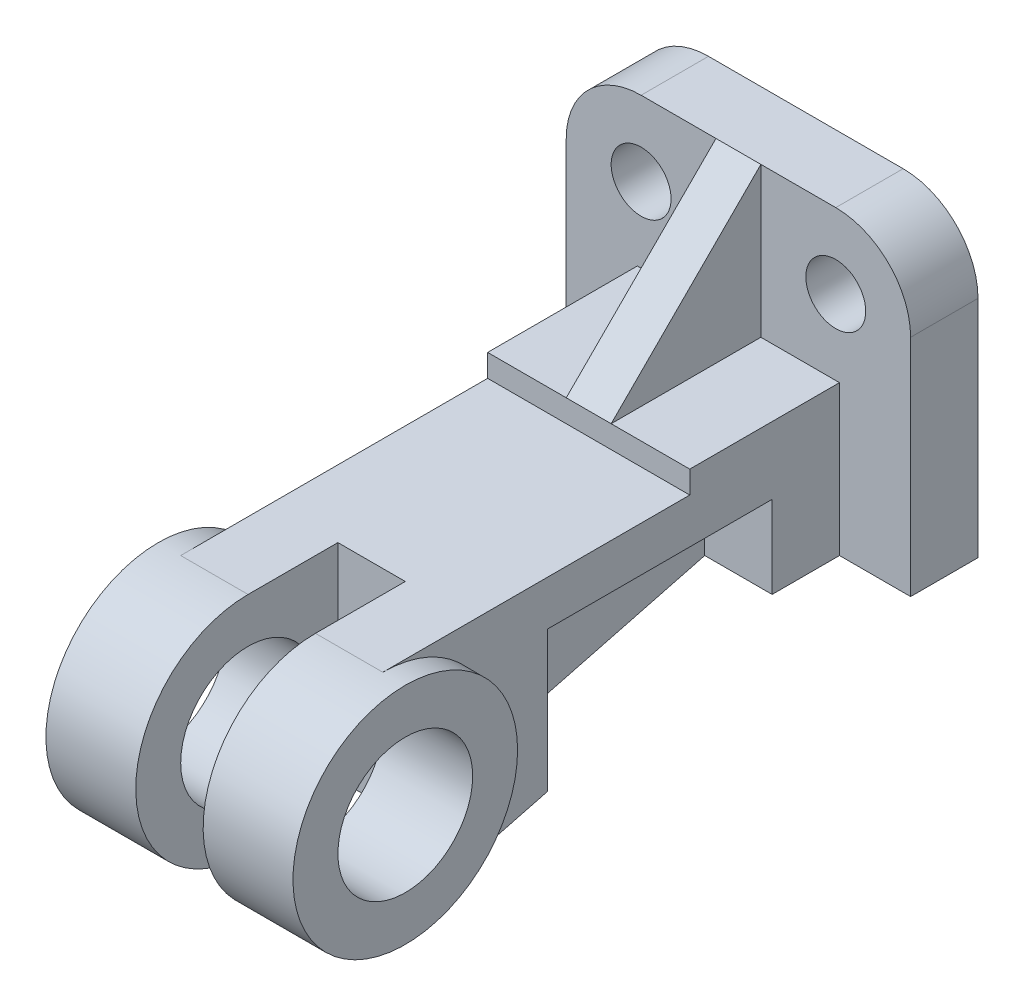
ISO-10303-21;
HEADER;
FILE_DESCRIPTION(('STEP AP214'),'2;1');
FILE_NAME('part.step','',(''),(''),'','','');
FILE_SCHEMA(('AUTOMOTIVE_DESIGN { 1 0 10303 214 1 1 1 1 }'));
ENDSEC;
DATA;
#1=APPLICATION_CONTEXT('core data for automotive mechanical design processes');
#2=APPLICATION_PROTOCOL_DEFINITION('international standard','automotive_design',2000,#1);
#3=PRODUCT_CONTEXT('',#1,'mechanical');
#4=PRODUCT('Part','Part','',(#3));
#5=PRODUCT_RELATED_PRODUCT_CATEGORY('part','',(#4));
#6=PRODUCT_DEFINITION_FORMATION('','',#4);
#7=PRODUCT_DEFINITION_CONTEXT('part definition',#1,'design');
#8=PRODUCT_DEFINITION('design','',#6,#7);
#9=PRODUCT_DEFINITION_SHAPE('','',#8);
#10=(LENGTH_UNIT() NAMED_UNIT(*) SI_UNIT(.MILLI.,.METRE.));
#11=(NAMED_UNIT(*) PLANE_ANGLE_UNIT() SI_UNIT($,.RADIAN.));
#12=(NAMED_UNIT(*) SI_UNIT($,.STERADIAN.) SOLID_ANGLE_UNIT());
#13=UNCERTAINTY_MEASURE_WITH_UNIT(LENGTH_MEASURE(1.E-05),#10,'distance_accuracy_value','');
#14=(GEOMETRIC_REPRESENTATION_CONTEXT(3) GLOBAL_UNCERTAINTY_ASSIGNED_CONTEXT((#13)) GLOBAL_UNIT_ASSIGNED_CONTEXT((#10,
#11,#12)) REPRESENTATION_CONTEXT('',''));
#15=CARTESIAN_POINT('',(0.,0.,0.));
#16=DIRECTION('',(0.,0.,1.));
#17=DIRECTION('',(1.,0.,0.));
#18=AXIS2_PLACEMENT_3D('',#15,#16,#17);
#19=CARTESIAN_POINT('',(27.,0.,26.));
#20=DIRECTION('',(0.,0.,1.));
#21=DIRECTION('',(1.,0.,0.));
#22=AXIS2_PLACEMENT_3D('',#19,#20,#21);
#23=PLANE('',#22);
#24=DIRECTION('',(0.,-1.,0.));
#25=VECTOR('',#24,1.);
#26=CARTESIAN_POINT('',(9.,-19.5735131149187,26.));
#27=LINE('',#26,#25);
#28=CARTESIAN_POINT('',(9.,18.,26.));
#29=VERTEX_POINT('',#28);
#30=CARTESIAN_POINT('',(9.,-19.5735131149187,26.));
#31=VERTEX_POINT('',#30);
#32=EDGE_CURVE('E64',#29,#31,#27,.T.);
#33=ORIENTED_EDGE('',*,*,#32,.F.);
#34=DIRECTION('',(-1.,0.,0.));
#35=VECTOR('',#34,1.);
#36=CARTESIAN_POINT('',(27.,18.,26.));
#37=LINE('',#36,#35);
#38=CARTESIAN_POINT('',(27.,18.,26.));
#39=VERTEX_POINT('',#38);
#40=EDGE_CURVE('E243',#39,#29,#37,.T.);
#41=ORIENTED_EDGE('',*,*,#40,.F.);
#42=DIRECTION('',(0.,1.,0.));
#43=VECTOR('',#42,1.);
#44=CARTESIAN_POINT('',(27.,0.,26.));
#45=LINE('',#44,#43);
#46=CARTESIAN_POINT('',(27.,-19.5735131149187,26.));
#47=VERTEX_POINT('',#46);
#48=EDGE_CURVE('E347',#47,#39,#45,.T.);
#49=ORIENTED_EDGE('',*,*,#48,.F.);
#50=DIRECTION('',(-1.,0.,0.));
#51=VECTOR('',#50,1.);
#52=CARTESIAN_POINT('',(27.,-19.5735131149187,26.));
#53=LINE('',#52,#51);
#54=EDGE_CURVE('E411',#47,#31,#53,.T.);
#55=ORIENTED_EDGE('',*,*,#54,.T.);
#56=EDGE_LOOP('',(#33,#41,#49,#55));
#57=FACE_BOUND('',#56,.T.);
#58=ADVANCED_FACE('F41',(#57),#23,.F.);
#59=CARTESIAN_POINT('',(27.,18.,0.));
#60=DIRECTION('',(0.,1.,0.));
#61=DIRECTION('',(0.,0.,1.));
#62=AXIS2_PLACEMENT_3D('',#59,#60,#61);
#63=PLANE('',#62);
#64=DIRECTION('',(0.,0.,1.));
#65=VECTOR('',#64,1.);
#66=CARTESIAN_POINT('',(9.,18.,26.));
#67=LINE('',#66,#65);
#68=CARTESIAN_POINT('',(9.,18.,-34.));
#69=VERTEX_POINT('',#68);
#70=EDGE_CURVE('E242',#69,#29,#67,.T.);
#71=ORIENTED_EDGE('',*,*,#70,.F.);
#72=DIRECTION('',(-1.,0.,0.));
#73=VECTOR('',#72,1.);
#74=CARTESIAN_POINT('',(27.,18.,-34.));
#75=LINE('',#74,#73);
#76=CARTESIAN_POINT('',(27.,18.,-34.));
#77=VERTEX_POINT('',#76);
#78=EDGE_CURVE('E230',#77,#69,#75,.T.);
#79=ORIENTED_EDGE('',*,*,#78,.F.);
#80=DIRECTION('',(0.,0.,-1.));
#81=VECTOR('',#80,1.);
#82=CARTESIAN_POINT('',(27.,18.,0.));
#83=LINE('',#82,#81);
#84=EDGE_CURVE('E346',#39,#77,#83,.T.);
#85=ORIENTED_EDGE('',*,*,#84,.F.);
#86=ORIENTED_EDGE('',*,*,#40,.T.);
#87=EDGE_LOOP('',(#71,#79,#85,#86));
#88=FACE_BOUND('',#87,.T.);
#89=ADVANCED_FACE('F245',(#88),#63,.F.);
#90=CARTESIAN_POINT('',(27.,0.,-34.));
#91=DIRECTION('',(0.,0.,-1.));
#92=DIRECTION('',(0.,1.,0.));
#93=AXIS2_PLACEMENT_3D('',#90,#91,#92);
#94=PLANE('',#93);
#95=DIRECTION('',(0.,1.,0.));
#96=VECTOR('',#95,1.);
#97=CARTESIAN_POINT('',(9.,18.,-34.));
#98=LINE('',#97,#96);
#99=CARTESIAN_POINT('',(9.,-3.99999999999996,-34.));
#100=VERTEX_POINT('',#99);
#101=EDGE_CURVE('E235',#100,#69,#98,.T.);
#102=ORIENTED_EDGE('',*,*,#101,.F.);
#103=DIRECTION('',(-1.,0.,0.));
#104=VECTOR('',#103,1.);
#105=CARTESIAN_POINT('',(27.,-3.99999999999996,-34.));
#106=LINE('',#105,#104);
#107=CARTESIAN_POINT('',(27.,-3.99999999999996,-34.));
#108=VERTEX_POINT('',#107);
#109=EDGE_CURVE('E410',#108,#100,#106,.T.);
#110=ORIENTED_EDGE('',*,*,#109,.F.);
#111=DIRECTION('',(0.,-1.,0.));
#112=VECTOR('',#111,1.);
#113=CARTESIAN_POINT('',(27.,0.,-34.));
#114=LINE('',#113,#112);
#115=EDGE_CURVE('E233',#77,#108,#114,.T.);
#116=ORIENTED_EDGE('',*,*,#115,.F.);
#117=ORIENTED_EDGE('',*,*,#78,.T.);
#118=EDGE_LOOP('',(#102,#110,#116,#117));
#119=FACE_BOUND('',#118,.T.);
#120=ADVANCED_FACE('F229',(#119),#94,.F.);
#121=CARTESIAN_POINT('',(46.,0.,-52.));
#122=DIRECTION('',(0.,0.,-1.));
#123=DIRECTION('',(0.,1.,0.));
#124=AXIS2_PLACEMENT_3D('',#121,#122,#123);
#125=PLANE('',#124);
#126=CARTESIAN_POINT('',(-26.,56.,-52.));
#127=DIRECTION('',(0.,0.,1.));
#128=DIRECTION('',(1.,0.,0.));
#129=AXIS2_PLACEMENT_3D('',#126,#127,#128);
#130=CIRCLE('',#129,8.);
#131=CARTESIAN_POINT('',(-18.,56.,-52.));
#132=VERTEX_POINT('',#131);
#133=EDGE_CURVE('E320',#132,#132,#130,.T.);
#134=ORIENTED_EDGE('',*,*,#133,.F.);
#135=EDGE_LOOP('',(#134));
#136=FACE_BOUND('',#135,.T.);
#137=DIRECTION('',(0.,-1.,0.));
#138=VECTOR('',#137,1.);
#139=CARTESIAN_POINT('',(-6.,0.,-52.));
#140=LINE('',#139,#138);
#141=CARTESIAN_POINT('',(-6.,76.0000000000001,-52.));
#142=VERTEX_POINT('',#141);
#143=CARTESIAN_POINT('',(-6.,36.,-52.));
#144=VERTEX_POINT('',#143);
#145=EDGE_CURVE('E282',#142,#144,#140,.T.);
#146=ORIENTED_EDGE('',*,*,#145,.F.);
#147=DIRECTION('',(-1.,0.,0.));
#148=VECTOR('',#147,1.);
#149=CARTESIAN_POINT('',(46.,76.0000000000001,-52.));
#150=LINE('',#149,#148);
#151=CARTESIAN_POINT('',(-26.,76.0000000000001,-52.));
#152=VERTEX_POINT('',#151);
#153=EDGE_CURVE('E426',#142,#152,#150,.T.);
#154=ORIENTED_EDGE('',*,*,#153,.T.);
#155=CARTESIAN_POINT('',(-26.,56.,-52.));
#156=DIRECTION('',(0.,0.,-1.));
#157=DIRECTION('',(0.,1.,0.));
#158=AXIS2_PLACEMENT_3D('',#155,#156,#157);
#159=CIRCLE('',#158,20.);
#160=CARTESIAN_POINT('',(-46.,56.,-52.));
#161=VERTEX_POINT('',#160);
#162=EDGE_CURVE('E458',#152,#161,#159,.F.);
#163=ORIENTED_EDGE('',*,*,#162,.T.);
#164=DIRECTION('',(0.,-1.,0.));
#165=VECTOR('',#164,1.);
#166=CARTESIAN_POINT('',(-46.,0.,-52.));
#167=LINE('',#166,#165);
#168=CARTESIAN_POINT('',(-46.,-3.99999999999995,-52.));
#169=VERTEX_POINT('',#168);
#170=EDGE_CURVE('E417',#161,#169,#167,.T.);
#171=ORIENTED_EDGE('',*,*,#170,.T.);
#172=DIRECTION('',(-1.,0.,0.));
#173=VECTOR('',#172,1.);
#174=CARTESIAN_POINT('',(46.,-3.99999999999995,-52.));
#175=LINE('',#174,#173);
#176=CARTESIAN_POINT('',(-27.,-3.99999999999995,-52.));
#177=VERTEX_POINT('',#176);
#178=EDGE_CURVE('E439',#177,#169,#175,.T.);
#179=ORIENTED_EDGE('',*,*,#178,.F.);
#180=DIRECTION('',(0.,-1.,0.));
#181=VECTOR('',#180,1.);
#182=CARTESIAN_POINT('',(-27.,0.,-52.));
#183=LINE('',#182,#181);
#184=CARTESIAN_POINT('',(-27.,36.,-52.));
#185=VERTEX_POINT('',#184);
#186=EDGE_CURVE('E385',#185,#177,#183,.T.);
#187=ORIENTED_EDGE('',*,*,#186,.F.);
#188=DIRECTION('',(-1.,0.,0.));
#189=VECTOR('',#188,1.);
#190=CARTESIAN_POINT('',(27.,36.,-52.));
#191=LINE('',#190,#189);
#192=EDGE_CURVE('E405',#144,#185,#191,.T.);
#193=ORIENTED_EDGE('',*,*,#192,.F.);
#194=EDGE_LOOP('',(#146,#154,#163,#171,#179,#187,#193));
#195=FACE_BOUND('',#194,.T.);
#196=ADVANCED_FACE('F519',(#136,#195),#125,.F.);
#197=CARTESIAN_POINT('',(27.,35.9999999999999,0.));
#198=DIRECTION('',(0.,1.,0.));
#199=DIRECTION('',(0.,0.,1.));
#200=AXIS2_PLACEMENT_3D('',#197,#198,#199);
#201=PLANE('',#200);
#202=DIRECTION('',(-1.,0.,0.));
#203=VECTOR('',#202,1.);
#204=CARTESIAN_POINT('',(27.,35.9999999999999,-12.));
#205=LINE('',#204,#203);
#206=CARTESIAN_POINT('',(-6.,35.9999999999999,-12.));
#207=VERTEX_POINT('',#206);
#208=CARTESIAN_POINT('',(-27.,35.9999999999999,-12.));
#209=VERTEX_POINT('',#208);
#210=EDGE_CURVE('E397',#207,#209,#205,.T.);
#211=ORIENTED_EDGE('',*,*,#210,.F.);
#212=DIRECTION('',(0.,0.,-1.));
#213=VECTOR('',#212,1.);
#214=CARTESIAN_POINT('',(-6.,35.9999999999999,0.));
#215=LINE('',#214,#213);
#216=EDGE_CURVE('E279',#207,#144,#215,.T.);
#217=ORIENTED_EDGE('',*,*,#216,.T.);
#218=ORIENTED_EDGE('',*,*,#192,.T.);
#219=DIRECTION('',(0.,0.,-1.));
#220=VECTOR('',#219,1.);
#221=CARTESIAN_POINT('',(-27.,35.9999999999999,0.));
#222=LINE('',#221,#220);
#223=EDGE_CURVE('E384',#209,#185,#222,.T.);
#224=ORIENTED_EDGE('',*,*,#223,.F.);
#225=EDGE_LOOP('',(#211,#217,#218,#224));
#226=FACE_BOUND('',#225,.T.);
#227=ADVANCED_FACE('F515',(#226),#201,.T.);
#228=CARTESIAN_POINT('',(33.,0.,70.));
#229=DIRECTION('',(-1.,0.,0.));
#230=DIRECTION('',(0.,0.,1.));
#231=AXIS2_PLACEMENT_3D('',#228,#229,#230);
#232=CYLINDRICAL_SURFACE('',#231,18.);
#233=CARTESIAN_POINT('',(-9.,0.,70.));
#234=DIRECTION('',(-1.,0.,0.));
#235=DIRECTION('',(0.,0.,1.));
#236=AXIS2_PLACEMENT_3D('',#233,#234,#235);
#237=CIRCLE('',#236,18.);
#238=CARTESIAN_POINT('',(-9.,0.,88.));
#239=VERTEX_POINT('',#238);
#240=EDGE_CURVE('E313',#239,#239,#237,.T.);
#241=ORIENTED_EDGE('',*,*,#240,.F.);
#242=EDGE_LOOP('',(#241));
#243=FACE_BOUND('',#242,.T.);
#244=CARTESIAN_POINT('',(-33.,0.,70.));
#245=DIRECTION('',(1.,0.,0.));
#246=DIRECTION('',(0.,0.,-1.));
#247=AXIS2_PLACEMENT_3D('',#244,#245,#246);
#248=CIRCLE('',#247,18.);
#249=CARTESIAN_POINT('',(-33.,0.,52.));
#250=VERTEX_POINT('',#249);
#251=EDGE_CURVE('E319',#250,#250,#248,.T.);
#252=ORIENTED_EDGE('',*,*,#251,.F.);
#253=EDGE_LOOP('',(#252));
#254=FACE_BOUND('',#253,.T.);
#255=ADVANCED_FACE('F606',(#243,#254),#232,.F.);
#256=CARTESIAN_POINT('',(33.,0.,70.));
#257=DIRECTION('',(-1.,0.,0.));
#258=DIRECTION('',(0.,0.,1.));
#259=AXIS2_PLACEMENT_3D('',#256,#257,#258);
#260=CYLINDRICAL_SURFACE('',#259,30.);
#261=CARTESIAN_POINT('',(33.,0.,70.));
#262=DIRECTION('',(1.,0.,0.));
#263=DIRECTION('',(0.,0.,-1.));
#264=AXIS2_PLACEMENT_3D('',#261,#262,#263);
#265=CIRCLE('',#264,30.);
#266=CARTESIAN_POINT('',(33.,0.,40.));
#267=VERTEX_POINT('',#266);
#268=EDGE_CURVE('E335',#267,#267,#265,.T.);
#269=ORIENTED_EDGE('',*,*,#268,.F.);
#270=EDGE_LOOP('',(#269));
#271=FACE_BOUND('',#270,.T.);
#272=DIRECTION('',(-1.,0.,0.));
#273=VECTOR('',#272,1.);
#274=CARTESIAN_POINT('',(27.,30.,70.));
#275=LINE('',#274,#273);
#276=CARTESIAN_POINT('',(27.,30.,70.));
#277=VERTEX_POINT('',#276);
#278=CARTESIAN_POINT('',(9.00000000000001,30.,70.));
#279=VERTEX_POINT('',#278);
#280=EDGE_CURVE('E393',#277,#279,#275,.T.);
#281=ORIENTED_EDGE('',*,*,#280,.T.);
#282=CARTESIAN_POINT('',(9.00000000000001,0.,70.));
#283=DIRECTION('',(1.,0.,0.));
#284=DIRECTION('',(0.,0.,-1.));
#285=AXIS2_PLACEMENT_3D('',#282,#283,#284);
#286=CIRCLE('',#285,30.);
#287=CARTESIAN_POINT('',(9.00000000000001,-29.0377945423184,62.4629920977815));
#288=VERTEX_POINT('',#287);
#289=EDGE_CURVE('E464',#279,#288,#286,.T.);
#290=ORIENTED_EDGE('',*,*,#289,.T.);
#291=DIRECTION('',(-1.,0.,0.));
#292=VECTOR('',#291,1.);
#293=CARTESIAN_POINT('',(27.,-29.0377945423184,62.4629920977815));
#294=LINE('',#293,#292);
#295=CARTESIAN_POINT('',(27.,-29.0377945423184,62.4629920977815));
#296=VERTEX_POINT('',#295);
#297=EDGE_CURVE('E413',#296,#288,#294,.T.);
#298=ORIENTED_EDGE('',*,*,#297,.F.);
#299=CARTESIAN_POINT('',(27.,0.,70.));
#300=DIRECTION('',(1.,0.,0.));
#301=DIRECTION('',(0.,0.,-1.));
#302=AXIS2_PLACEMENT_3D('',#299,#300,#301);
#303=CIRCLE('',#302,30.);
#304=EDGE_CURVE('E341',#296,#277,#303,.T.);
#305=ORIENTED_EDGE('',*,*,#304,.T.);
#306=EDGE_LOOP('',(#281,#290,#298,#305));
#307=FACE_BOUND('',#306,.T.);
#308=ADVANCED_FACE('F496',(#271,#307),#260,.T.);
#309=CARTESIAN_POINT('',(26.,56.,-52.));
#310=DIRECTION('',(0.,0.,1.));
#311=DIRECTION('',(1.,0.,0.));
#312=AXIS2_PLACEMENT_3D('',#309,#310,#311);
#313=CIRCLE('',#312,8.);
#314=CARTESIAN_POINT('',(34.,56.,-52.));
#315=VERTEX_POINT('',#314);
#316=EDGE_CURVE('E316',#315,#315,#313,.T.);
#317=ORIENTED_EDGE('',*,*,#316,.F.);
#318=EDGE_LOOP('',(#317));
#319=FACE_BOUND('',#318,.T.);
#320=CARTESIAN_POINT('',(26.,76.0000000000001,-52.));
#321=VERTEX_POINT('',#320);
#322=CARTESIAN_POINT('',(6.,76.0000000000001,-52.));
#323=VERTEX_POINT('',#322);
#324=EDGE_CURVE('E433',#321,#323,#150,.T.);
#325=ORIENTED_EDGE('',*,*,#324,.T.);
#326=DIRECTION('',(0.,-1.,0.));
#327=VECTOR('',#326,1.);
#328=CARTESIAN_POINT('',(6.,0.,-52.));
#329=LINE('',#328,#327);
#330=CARTESIAN_POINT('',(6.,36.,-52.));
#331=VERTEX_POINT('',#330);
#332=EDGE_CURVE('E281',#323,#331,#329,.T.);
#333=ORIENTED_EDGE('',*,*,#332,.T.);
#334=CARTESIAN_POINT('',(27.,36.,-52.));
#335=VERTEX_POINT('',#334);
#336=EDGE_CURVE('E401',#335,#331,#191,.T.);
#337=ORIENTED_EDGE('',*,*,#336,.F.);
#338=DIRECTION('',(0.,-1.,0.));
#339=VECTOR('',#338,1.);
#340=CARTESIAN_POINT('',(27.,0.,-52.));
#341=LINE('',#340,#339);
#342=CARTESIAN_POINT('',(27.,-3.99999999999995,-52.));
#343=VERTEX_POINT('',#342);
#344=EDGE_CURVE('E353',#335,#343,#341,.T.);
#345=ORIENTED_EDGE('',*,*,#344,.T.);
#346=CARTESIAN_POINT('',(46.,-3.99999999999995,-52.));
#347=VERTEX_POINT('',#346);
#348=EDGE_CURVE('E442',#347,#343,#175,.T.);
#349=ORIENTED_EDGE('',*,*,#348,.F.);
#350=DIRECTION('',(0.,-1.,0.));
#351=VECTOR('',#350,1.);
#352=CARTESIAN_POINT('',(46.,0.,-52.));
#353=LINE('',#352,#351);
#354=CARTESIAN_POINT('',(46.,56.,-52.));
#355=VERTEX_POINT('',#354);
#356=EDGE_CURVE('E416',#355,#347,#353,.T.);
#357=ORIENTED_EDGE('',*,*,#356,.F.);
#358=CARTESIAN_POINT('',(26.,56.,-52.));
#359=DIRECTION('',(0.,0.,-1.));
#360=DIRECTION('',(0.,1.,0.));
#361=AXIS2_PLACEMENT_3D('',#358,#359,#360);
#362=CIRCLE('',#361,20.);
#363=EDGE_CURVE('E456',#355,#321,#362,.F.);
#364=ORIENTED_EDGE('',*,*,#363,.T.);
#365=EDGE_LOOP('',(#325,#333,#337,#345,#349,#357,#364));
#366=FACE_BOUND('',#365,.T.);
#367=ADVANCED_FACE('F545',(#319,#366),#125,.F.);
#368=CARTESIAN_POINT('',(46.,-3.99999999999995,0.));
#369=DIRECTION('',(0.,1.,0.));
#370=DIRECTION('',(0.,0.,1.));
#371=AXIS2_PLACEMENT_3D('',#368,#369,#370);
#372=PLANE('',#371);
#373=ORIENTED_EDGE('',*,*,#109,.T.);
#374=DIRECTION('',(-1.,0.,0.));
#375=VECTOR('',#374,1.);
#376=CARTESIAN_POINT('',(9.,-3.99999999999996,-34.));
#377=LINE('',#376,#375);
#378=CARTESIAN_POINT('',(-9.,-3.99999999999996,-34.));
#379=VERTEX_POINT('',#378);
#380=EDGE_CURVE('E241',#100,#379,#377,.T.);
#381=ORIENTED_EDGE('',*,*,#380,.T.);
#382=CARTESIAN_POINT('',(-27.,-3.99999999999996,-34.));
#383=VERTEX_POINT('',#382);
#384=EDGE_CURVE('E407',#379,#383,#106,.T.);
#385=ORIENTED_EDGE('',*,*,#384,.T.);
#386=DIRECTION('',(0.,0.,-1.));
#387=VECTOR('',#386,1.);
#388=CARTESIAN_POINT('',(-27.,-3.99999999999997,0.));
#389=LINE('',#388,#387);
#390=EDGE_CURVE('E379',#383,#177,#389,.T.);
#391=ORIENTED_EDGE('',*,*,#390,.T.);
#392=ORIENTED_EDGE('',*,*,#178,.T.);
#393=DIRECTION('',(0.,0.,-1.));
#394=VECTOR('',#393,1.);
#395=CARTESIAN_POINT('',(-46.,-3.99999999999995,0.));
#396=LINE('',#395,#394);
#397=CARTESIAN_POINT('',(-46.,-3.99999999999995,-70.));
#398=VERTEX_POINT('',#397);
#399=EDGE_CURVE('E428',#169,#398,#396,.T.);
#400=ORIENTED_EDGE('',*,*,#399,.T.);
#401=DIRECTION('',(-1.,0.,0.));
#402=VECTOR('',#401,1.);
#403=CARTESIAN_POINT('',(46.,-3.99999999999995,-70.));
#404=LINE('',#403,#402);
#405=CARTESIAN_POINT('',(46.,-3.99999999999995,-70.));
#406=VERTEX_POINT('',#405);
#407=EDGE_CURVE('E437',#406,#398,#404,.T.);
#408=ORIENTED_EDGE('',*,*,#407,.F.);
#409=DIRECTION('',(0.,0.,-1.));
#410=VECTOR('',#409,1.);
#411=CARTESIAN_POINT('',(46.,-3.99999999999995,0.));
#412=LINE('',#411,#410);
#413=EDGE_CURVE('E419',#347,#406,#412,.T.);
#414=ORIENTED_EDGE('',*,*,#413,.F.);
#415=ORIENTED_EDGE('',*,*,#348,.T.);
#416=DIRECTION('',(0.,0.,-1.));
#417=VECTOR('',#416,1.);
#418=CARTESIAN_POINT('',(27.,-3.99999999999997,0.));
#419=LINE('',#418,#417);
#420=EDGE_CURVE('E352',#108,#343,#419,.T.);
#421=ORIENTED_EDGE('',*,*,#420,.F.);
#422=EDGE_LOOP('',(#373,#381,#385,#391,#392,#400,#408,#414,#415,#421));
#423=FACE_BOUND('',#422,.T.);
#424=ADVANCED_FACE('F523',(#423),#372,.F.);
#425=CARTESIAN_POINT('',(46.,0.,-70.));
#426=DIRECTION('',(0.,0.,-1.));
#427=DIRECTION('',(0.,1.,0.));
#428=AXIS2_PLACEMENT_3D('',#425,#426,#427);
#429=PLANE('',#428);
#430=ORIENTED_EDGE('',*,*,#407,.T.);
#431=DIRECTION('',(0.,-1.,0.));
#432=VECTOR('',#431,1.);
#433=CARTESIAN_POINT('',(-46.,0.,-70.));
#434=LINE('',#433,#432);
#435=CARTESIAN_POINT('',(-46.,56.,-70.));
#436=VERTEX_POINT('',#435);
#437=EDGE_CURVE('E423',#436,#398,#434,.T.);
#438=ORIENTED_EDGE('',*,*,#437,.F.);
#439=CARTESIAN_POINT('',(-26.,56.,-70.));
#440=DIRECTION('',(0.,0.,-1.));
#441=DIRECTION('',(0.,1.,0.));
#442=AXIS2_PLACEMENT_3D('',#439,#440,#441);
#443=CIRCLE('',#442,20.);
#444=CARTESIAN_POINT('',(-26.,76.0000000000001,-70.));
#445=VERTEX_POINT('',#444);
#446=EDGE_CURVE('E449',#436,#445,#443,.T.);
#447=ORIENTED_EDGE('',*,*,#446,.T.);
#448=DIRECTION('',(-1.,0.,0.));
#449=VECTOR('',#448,1.);
#450=CARTESIAN_POINT('',(46.,76.0000000000001,-70.));
#451=LINE('',#450,#449);
#452=CARTESIAN_POINT('',(26.,76.0000000000001,-70.));
#453=VERTEX_POINT('',#452);
#454=EDGE_CURVE('E436',#453,#445,#451,.T.);
#455=ORIENTED_EDGE('',*,*,#454,.F.);
#456=CARTESIAN_POINT('',(26.,56.,-70.));
#457=DIRECTION('',(0.,0.,-1.));
#458=DIRECTION('',(0.,1.,0.));
#459=AXIS2_PLACEMENT_3D('',#456,#457,#458);
#460=CIRCLE('',#459,20.);
#461=CARTESIAN_POINT('',(46.,56.,-70.));
#462=VERTEX_POINT('',#461);
#463=EDGE_CURVE('E450',#453,#462,#460,.T.);
#464=ORIENTED_EDGE('',*,*,#463,.T.);
#465=DIRECTION('',(0.,-1.,0.));
#466=VECTOR('',#465,1.);
#467=CARTESIAN_POINT('',(46.,0.,-70.));
#468=LINE('',#467,#466);
#469=EDGE_CURVE('E424',#462,#406,#468,.T.);
#470=ORIENTED_EDGE('',*,*,#469,.T.);
#471=EDGE_LOOP('',(#430,#438,#447,#455,#464,#470));
#472=FACE_BOUND('',#471,.T.);
#473=CARTESIAN_POINT('',(26.,56.,-70.));
#474=DIRECTION('',(0.,0.,-1.));
#475=DIRECTION('',(0.,1.,0.));
#476=AXIS2_PLACEMENT_3D('',#473,#474,#475);
#477=CIRCLE('',#476,8.);
#478=CARTESIAN_POINT('',(26.,64.0000000000001,-70.));
#479=VERTEX_POINT('',#478);
#480=EDGE_CURVE('E322',#479,#479,#477,.F.);
#481=ORIENTED_EDGE('',*,*,#480,.T.);
#482=EDGE_LOOP('',(#481));
#483=FACE_BOUND('',#482,.T.);
#484=CARTESIAN_POINT('',(-26.,56.,-70.));
#485=DIRECTION('',(0.,0.,-1.));
#486=DIRECTION('',(0.,1.,0.));
#487=AXIS2_PLACEMENT_3D('',#484,#485,#486);
#488=CIRCLE('',#487,8.);
#489=CARTESIAN_POINT('',(-26.,64.0000000000001,-70.));
#490=VERTEX_POINT('',#489);
#491=EDGE_CURVE('E321',#490,#490,#488,.F.);
#492=ORIENTED_EDGE('',*,*,#491,.T.);
#493=EDGE_LOOP('',(#492));
#494=FACE_BOUND('',#493,.T.);
#495=ADVANCED_FACE('F533',(#472,#483,#494),#429,.T.);
#496=CARTESIAN_POINT('',(46.,76.0000000000001,0.));
#497=DIRECTION('',(0.,1.,0.));
#498=DIRECTION('',(0.,0.,1.));
#499=AXIS2_PLACEMENT_3D('',#496,#497,#498);
#500=PLANE('',#499);
#501=ORIENTED_EDGE('',*,*,#454,.T.);
#502=DIRECTION('',(0.,0.,-1.));
#503=VECTOR('',#502,1.);
#504=CARTESIAN_POINT('',(-26.,76.0000000000001,-52.));
#505=LINE('',#504,#503);
#506=EDGE_CURVE('E454',#445,#152,#505,.F.);
#507=ORIENTED_EDGE('',*,*,#506,.T.);
#508=ORIENTED_EDGE('',*,*,#153,.F.);
#509=DIRECTION('',(0.,0.,-1.));
#510=VECTOR('',#509,1.);
#511=CARTESIAN_POINT('',(-6.,76.0000000000001,15.));
#512=LINE('',#511,#510);
#513=CARTESIAN_POINT('',(-6.,76.0000000000001,-51.9999));
#514=VERTEX_POINT('',#513);
#515=EDGE_CURVE('E266',#142,#514,#512,.F.);
#516=ORIENTED_EDGE('',*,*,#515,.T.);
#517=DIRECTION('',(1.,0.,0.));
#518=VECTOR('',#517,1.);
#519=CARTESIAN_POINT('',(0.,76.0000000000001,-51.9999));
#520=LINE('',#519,#518);
#521=CARTESIAN_POINT('',(6.,76.0000000000001,-51.9999));
#522=VERTEX_POINT('',#521);
#523=EDGE_CURVE('E272',#514,#522,#520,.T.);
#524=ORIENTED_EDGE('',*,*,#523,.T.);
#525=DIRECTION('',(0.,0.,-1.));
#526=VECTOR('',#525,1.);
#527=CARTESIAN_POINT('',(6.,76.0000000000001,15.));
#528=LINE('',#527,#526);
#529=EDGE_CURVE('E270',#323,#522,#528,.F.);
#530=ORIENTED_EDGE('',*,*,#529,.F.);
#531=ORIENTED_EDGE('',*,*,#324,.F.);
#532=DIRECTION('',(0.,0.,-1.));
#533=VECTOR('',#532,1.);
#534=CARTESIAN_POINT('',(26.,76.0000000000001,0.));
#535=LINE('',#534,#533);
#536=EDGE_CURVE('E455',#321,#453,#535,.T.);
#537=ORIENTED_EDGE('',*,*,#536,.T.);
#538=EDGE_LOOP('',(#501,#507,#508,#516,#524,#530,#531,#537));
#539=FACE_BOUND('',#538,.T.);
#540=ADVANCED_FACE('F553',(#539),#500,.T.);
#541=CARTESIAN_POINT('',(46.,0.,0.));
#542=DIRECTION('',(1.,0.,0.));
#543=DIRECTION('',(0.,0.,-1.));
#544=AXIS2_PLACEMENT_3D('',#541,#542,#543);
#545=PLANE('',#544);
#546=ORIENTED_EDGE('',*,*,#469,.F.);
#547=DIRECTION('',(0.,0.,-1.));
#548=VECTOR('',#547,1.);
#549=CARTESIAN_POINT('',(46.,56.,0.));
#550=LINE('',#549,#548);
#551=EDGE_CURVE('E465',#462,#355,#550,.F.);
#552=ORIENTED_EDGE('',*,*,#551,.T.);
#553=ORIENTED_EDGE('',*,*,#356,.T.);
#554=ORIENTED_EDGE('',*,*,#413,.T.);
#555=EDGE_LOOP('',(#546,#552,#553,#554));
#556=FACE_BOUND('',#555,.T.);
#557=ADVANCED_FACE('F558',(#556),#545,.T.);
#558=CARTESIAN_POINT('',(-46.,0.,0.));
#559=DIRECTION('',(1.,0.,0.));
#560=DIRECTION('',(0.,0.,-1.));
#561=AXIS2_PLACEMENT_3D('',#558,#559,#560);
#562=PLANE('',#561);
#563=ORIENTED_EDGE('',*,*,#170,.F.);
#564=DIRECTION('',(0.,0.,-1.));
#565=VECTOR('',#564,1.);
#566=CARTESIAN_POINT('',(-46.,56.,-70.));
#567=LINE('',#566,#565);
#568=EDGE_CURVE('E441',#161,#436,#567,.T.);
#569=ORIENTED_EDGE('',*,*,#568,.T.);
#570=ORIENTED_EDGE('',*,*,#437,.T.);
#571=ORIENTED_EDGE('',*,*,#399,.F.);
#572=EDGE_LOOP('',(#563,#569,#570,#571));
#573=FACE_BOUND('',#572,.T.);
#574=ADVANCED_FACE('F527',(#573),#562,.F.);
#575=CARTESIAN_POINT('',(27.,-12.0154988923277,-3.11872549303262));
#576=DIRECTION('',(0.,0.967926484743946,0.251233596740618));
#577=DIRECTION('',(0.,-0.251233596740618,0.967926484743946));
#578=AXIS2_PLACEMENT_3D('',#575,#576,#577);
#579=PLANE('',#578);
#580=DIRECTION('',(-1.,0.,0.));
#581=VECTOR('',#580,1.);
#582=CARTESIAN_POINT('',(27.,-24.764684153225,46.));
#583=LINE('',#582,#581);
#584=CARTESIAN_POINT('',(9.00000000000001,-24.764684153225,46.));
#585=VERTEX_POINT('',#584);
#586=CARTESIAN_POINT('',(-9.00000000000001,-24.764684153225,46.));
#587=VERTEX_POINT('',#586);
#588=EDGE_CURVE('E314',#585,#587,#583,.T.);
#589=ORIENTED_EDGE('',*,*,#588,.T.);
#590=DIRECTION('',(0.,-0.251233596740618,0.967926484743946));
#591=VECTOR('',#590,1.);
#592=CARTESIAN_POINT('',(-9.00000000000001,-12.0154988923277,-3.11872549303261));
#593=LINE('',#592,#591);
#594=CARTESIAN_POINT('',(-9.,-29.0377945423184,62.4629920977815));
#595=VERTEX_POINT('',#594);
#596=EDGE_CURVE('E306',#587,#595,#593,.T.);
#597=ORIENTED_EDGE('',*,*,#596,.T.);
#598=CARTESIAN_POINT('',(-27.,-29.0377945423184,62.4629920977815));
#599=VERTEX_POINT('',#598);
#600=EDGE_CURVE('E412',#595,#599,#294,.T.);
#601=ORIENTED_EDGE('',*,*,#600,.T.);
#602=DIRECTION('',(0.,0.251233596740618,-0.967926484743946));
#603=VECTOR('',#602,1.);
#604=CARTESIAN_POINT('',(-27.,-12.0154988923277,-3.11872549303262));
#605=LINE('',#604,#603);
#606=CARTESIAN_POINT('',(-27.,-19.5735131149187,26.));
#607=VERTEX_POINT('',#606);
#608=EDGE_CURVE('E366',#599,#607,#605,.T.);
#609=ORIENTED_EDGE('',*,*,#608,.T.);
#610=CARTESIAN_POINT('',(-9.,-19.5735131149187,26.));
#611=VERTEX_POINT('',#610);
#612=EDGE_CURVE('E406',#611,#607,#53,.T.);
#613=ORIENTED_EDGE('',*,*,#612,.F.);
#614=DIRECTION('',(0.,0.251233596740618,-0.967926484743946));
#615=VECTOR('',#614,1.);
#616=CARTESIAN_POINT('',(-9.,-19.5735131149187,26.));
#617=LINE('',#616,#615);
#618=EDGE_CURVE('E256',#611,#379,#617,.T.);
#619=ORIENTED_EDGE('',*,*,#618,.T.);
#620=ORIENTED_EDGE('',*,*,#380,.F.);
#621=DIRECTION('',(0.,0.251233596740618,-0.967926484743946));
#622=VECTOR('',#621,1.);
#623=CARTESIAN_POINT('',(9.,-19.5735131149187,26.));
#624=LINE('',#623,#622);
#625=EDGE_CURVE('E249',#31,#100,#624,.T.);
#626=ORIENTED_EDGE('',*,*,#625,.F.);
#627=ORIENTED_EDGE('',*,*,#54,.F.);
#628=DIRECTION('',(0.,0.251233596740618,-0.967926484743946));
#629=VECTOR('',#628,1.);
#630=CARTESIAN_POINT('',(27.,-12.0154988923277,-3.11872549303262));
#631=LINE('',#630,#629);
#632=EDGE_CURVE('E342',#296,#47,#631,.T.);
#633=ORIENTED_EDGE('',*,*,#632,.F.);
#634=ORIENTED_EDGE('',*,*,#297,.T.);
#635=DIRECTION('',(0.,0.251233596740618,-0.967926484743946));
#636=VECTOR('',#635,1.);
#637=CARTESIAN_POINT('',(9.00000000000001,-12.0154988923277,-3.11872549303262));
#638=LINE('',#637,#636);
#639=EDGE_CURVE('E299',#288,#585,#638,.T.);
#640=ORIENTED_EDGE('',*,*,#639,.T.);
#641=EDGE_LOOP('',(#589,#597,#601,#609,#613,#619,#620,#626,#627,#633,#634,#640));
#642=FACE_BOUND('',#641,.T.);
#643=ADVANCED_FACE('F487',(#642),#579,.F.);
#644=CARTESIAN_POINT('',(-9.,18.,26.));
#645=VERTEX_POINT('',#644);
#646=CARTESIAN_POINT('',(-27.,18.,26.));
#647=VERTEX_POINT('',#646);
#648=EDGE_CURVE('E240',#645,#647,#37,.T.);
#649=ORIENTED_EDGE('',*,*,#648,.F.);
#650=DIRECTION('',(0.,-1.,0.));
#651=VECTOR('',#650,1.);
#652=CARTESIAN_POINT('',(-9.,-19.5735131149187,26.));
#653=LINE('',#652,#651);
#654=EDGE_CURVE('E258',#645,#611,#653,.T.);
#655=ORIENTED_EDGE('',*,*,#654,.T.);
#656=ORIENTED_EDGE('',*,*,#612,.T.);
#657=DIRECTION('',(0.,1.,0.));
#658=VECTOR('',#657,1.);
#659=CARTESIAN_POINT('',(-27.,0.,26.));
#660=LINE('',#659,#658);
#661=EDGE_CURVE('E371',#607,#647,#660,.T.);
#662=ORIENTED_EDGE('',*,*,#661,.T.);
#663=EDGE_LOOP('',(#649,#655,#656,#662));
#664=FACE_BOUND('',#663,.T.);
#665=ADVANCED_FACE('F572',(#664),#23,.F.);
#666=CARTESIAN_POINT('',(-9.,18.,-34.));
#667=VERTEX_POINT('',#666);
#668=CARTESIAN_POINT('',(-27.,18.,-34.));
#669=VERTEX_POINT('',#668);
#670=EDGE_CURVE('E236',#667,#669,#75,.T.);
#671=ORIENTED_EDGE('',*,*,#670,.F.);
#672=DIRECTION('',(0.,0.,1.));
#673=VECTOR('',#672,1.);
#674=CARTESIAN_POINT('',(-9.,18.,26.));
#675=LINE('',#674,#673);
#676=EDGE_CURVE('E57',#667,#645,#675,.T.);
#677=ORIENTED_EDGE('',*,*,#676,.T.);
#678=ORIENTED_EDGE('',*,*,#648,.T.);
#679=DIRECTION('',(0.,0.,-1.));
#680=VECTOR('',#679,1.);
#681=CARTESIAN_POINT('',(-27.,18.,0.));
#682=LINE('',#681,#680);
#683=EDGE_CURVE('E372',#647,#669,#682,.T.);
#684=ORIENTED_EDGE('',*,*,#683,.T.);
#685=EDGE_LOOP('',(#671,#677,#678,#684));
#686=FACE_BOUND('',#685,.T.);
#687=ADVANCED_FACE('F580',(#686),#63,.F.);
#688=ORIENTED_EDGE('',*,*,#384,.F.);
#689=DIRECTION('',(0.,1.,0.));
#690=VECTOR('',#689,1.);
#691=CARTESIAN_POINT('',(-9.,18.,-34.));
#692=LINE('',#691,#690);
#693=EDGE_CURVE('E261',#379,#667,#692,.T.);
#694=ORIENTED_EDGE('',*,*,#693,.T.);
#695=ORIENTED_EDGE('',*,*,#670,.T.);
#696=DIRECTION('',(0.,-1.,0.));
#697=VECTOR('',#696,1.);
#698=CARTESIAN_POINT('',(-27.,0.,-34.));
#699=LINE('',#698,#697);
#700=EDGE_CURVE('E380',#669,#383,#699,.T.);
#701=ORIENTED_EDGE('',*,*,#700,.T.);
#702=EDGE_LOOP('',(#688,#694,#695,#701));
#703=FACE_BOUND('',#702,.T.);
#704=ADVANCED_FACE('F585',(#703),#94,.F.);
#705=DIRECTION('',(0.,0.,-1.));
#706=VECTOR('',#705,1.);
#707=CARTESIAN_POINT('',(6.,35.9999999999999,0.));
#708=LINE('',#707,#706);
#709=CARTESIAN_POINT('',(6.,36.,-12.));
#710=VERTEX_POINT('',#709);
#711=EDGE_CURVE('E283',#710,#331,#708,.T.);
#712=ORIENTED_EDGE('',*,*,#711,.F.);
#713=CARTESIAN_POINT('',(27.,35.9999999999999,-12.));
#714=VERTEX_POINT('',#713);
#715=EDGE_CURVE('E398',#714,#710,#205,.T.);
#716=ORIENTED_EDGE('',*,*,#715,.F.);
#717=DIRECTION('',(0.,0.,-1.));
#718=VECTOR('',#717,1.);
#719=CARTESIAN_POINT('',(27.,35.9999999999999,0.));
#720=LINE('',#719,#718);
#721=EDGE_CURVE('E356',#714,#335,#720,.T.);
#722=ORIENTED_EDGE('',*,*,#721,.T.);
#723=ORIENTED_EDGE('',*,*,#336,.T.);
#724=EDGE_LOOP('',(#712,#716,#722,#723));
#725=FACE_BOUND('',#724,.T.);
#726=ADVANCED_FACE('F550',(#725),#201,.T.);
#727=CARTESIAN_POINT('',(27.,0.,-12.));
#728=DIRECTION('',(0.,0.,1.));
#729=DIRECTION('',(0.,-1.,0.));
#730=AXIS2_PLACEMENT_3D('',#727,#728,#729);
#731=PLANE('',#730);
#732=ORIENTED_EDGE('',*,*,#715,.T.);
#733=DIRECTION('',(-1.,0.,0.));
#734=VECTOR('',#733,1.);
#735=CARTESIAN_POINT('',(27.,35.9999999999999,-12.));
#736=LINE('',#735,#734);
#737=EDGE_CURVE('E287',#710,#207,#736,.T.);
#738=ORIENTED_EDGE('',*,*,#737,.T.);
#739=ORIENTED_EDGE('',*,*,#210,.T.);
#740=DIRECTION('',(0.,1.,0.));
#741=VECTOR('',#740,1.);
#742=CARTESIAN_POINT('',(-27.,0.,-12.));
#743=LINE('',#742,#741);
#744=CARTESIAN_POINT('',(-27.,29.9999999999999,-12.));
#745=VERTEX_POINT('',#744);
#746=EDGE_CURVE('E389',#745,#209,#743,.T.);
#747=ORIENTED_EDGE('',*,*,#746,.F.);
#748=DIRECTION('',(-1.,0.,0.));
#749=VECTOR('',#748,1.);
#750=CARTESIAN_POINT('',(27.,29.9999999999999,-12.));
#751=LINE('',#750,#749);
#752=CARTESIAN_POINT('',(27.,29.9999999999999,-12.));
#753=VERTEX_POINT('',#752);
#754=EDGE_CURVE('E396',#753,#745,#751,.T.);
#755=ORIENTED_EDGE('',*,*,#754,.F.);
#756=DIRECTION('',(0.,1.,0.));
#757=VECTOR('',#756,1.);
#758=CARTESIAN_POINT('',(27.,0.,-12.));
#759=LINE('',#758,#757);
#760=EDGE_CURVE('E358',#753,#714,#759,.T.);
#761=ORIENTED_EDGE('',*,*,#760,.T.);
#762=EDGE_LOOP('',(#732,#738,#739,#747,#755,#761));
#763=FACE_BOUND('',#762,.T.);
#764=ADVANCED_FACE('F507',(#763),#731,.T.);
#765=CARTESIAN_POINT('',(27.,30.,0.));
#766=DIRECTION('',(0.,1.,0.));
#767=DIRECTION('',(0.,0.,1.));
#768=AXIS2_PLACEMENT_3D('',#765,#766,#767);
#769=PLANE('',#768);
#770=ORIENTED_EDGE('',*,*,#754,.T.);
#771=DIRECTION('',(0.,0.,-1.));
#772=VECTOR('',#771,1.);
#773=CARTESIAN_POINT('',(-27.,30.,0.));
#774=LINE('',#773,#772);
#775=CARTESIAN_POINT('',(-27.,30.,70.));
#776=VERTEX_POINT('',#775);
#777=EDGE_CURVE('E343',#776,#745,#774,.T.);
#778=ORIENTED_EDGE('',*,*,#777,.F.);
#779=CARTESIAN_POINT('',(-9.,30.,70.));
#780=VERTEX_POINT('',#779);
#781=EDGE_CURVE('E364',#780,#776,#275,.T.);
#782=ORIENTED_EDGE('',*,*,#781,.F.);
#783=DIRECTION('',(0.,0.,1.));
#784=VECTOR('',#783,1.);
#785=CARTESIAN_POINT('',(-9.00000000000001,30.,0.));
#786=LINE('',#785,#784);
#787=CARTESIAN_POINT('',(-9.00000000000001,30.,46.));
#788=VERTEX_POINT('',#787);
#789=EDGE_CURVE('E304',#788,#780,#786,.T.);
#790=ORIENTED_EDGE('',*,*,#789,.F.);
#791=DIRECTION('',(-1.,0.,0.));
#792=VECTOR('',#791,1.);
#793=CARTESIAN_POINT('',(27.,30.,46.));
#794=LINE('',#793,#792);
#795=CARTESIAN_POINT('',(9.00000000000001,30.,46.));
#796=VERTEX_POINT('',#795);
#797=EDGE_CURVE('E11',#796,#788,#794,.T.);
#798=ORIENTED_EDGE('',*,*,#797,.F.);
#799=DIRECTION('',(0.,0.,-1.));
#800=VECTOR('',#799,1.);
#801=CARTESIAN_POINT('',(9.00000000000001,30.,0.));
#802=LINE('',#801,#800);
#803=EDGE_CURVE('E293',#279,#796,#802,.T.);
#804=ORIENTED_EDGE('',*,*,#803,.F.);
#805=ORIENTED_EDGE('',*,*,#280,.F.);
#806=DIRECTION('',(0.,0.,-1.));
#807=VECTOR('',#806,1.);
#808=CARTESIAN_POINT('',(27.,30.,0.));
#809=LINE('',#808,#807);
#810=EDGE_CURVE('E362',#277,#753,#809,.T.);
#811=ORIENTED_EDGE('',*,*,#810,.T.);
#812=EDGE_LOOP('',(#770,#778,#782,#790,#798,#804,#805,#811));
#813=FACE_BOUND('',#812,.T.);
#814=ADVANCED_FACE('F477',(#813),#769,.T.);
#815=CARTESIAN_POINT('',(27.,0.,0.));
#816=DIRECTION('',(1.,0.,0.));
#817=DIRECTION('',(0.,0.,-1.));
#818=AXIS2_PLACEMENT_3D('',#815,#816,#817);
#819=PLANE('',#818);
#820=ORIENTED_EDGE('',*,*,#304,.F.);
#821=ORIENTED_EDGE('',*,*,#632,.T.);
#822=ORIENTED_EDGE('',*,*,#48,.T.);
#823=ORIENTED_EDGE('',*,*,#84,.T.);
#824=ORIENTED_EDGE('',*,*,#115,.T.);
#825=ORIENTED_EDGE('',*,*,#420,.T.);
#826=ORIENTED_EDGE('',*,*,#344,.F.);
#827=ORIENTED_EDGE('',*,*,#721,.F.);
#828=ORIENTED_EDGE('',*,*,#760,.F.);
#829=ORIENTED_EDGE('',*,*,#810,.F.);
#830=EDGE_LOOP('',(#820,#821,#822,#823,#824,#825,#826,#827,#828,#829));
#831=FACE_BOUND('',#830,.T.);
#832=ADVANCED_FACE('F503',(#831),#819,.T.);
#833=CARTESIAN_POINT('',(-27.,0.,0.));
#834=DIRECTION('',(1.,0.,0.));
#835=DIRECTION('',(0.,0.,-1.));
#836=AXIS2_PLACEMENT_3D('',#833,#834,#835);
#837=PLANE('',#836);
#838=CARTESIAN_POINT('',(-27.,0.,70.));
#839=DIRECTION('',(1.,0.,0.));
#840=DIRECTION('',(0.,0.,-1.));
#841=AXIS2_PLACEMENT_3D('',#838,#839,#840);
#842=CIRCLE('',#841,30.);
#843=EDGE_CURVE('E337',#599,#776,#842,.T.);
#844=ORIENTED_EDGE('',*,*,#843,.T.);
#845=ORIENTED_EDGE('',*,*,#777,.T.);
#846=ORIENTED_EDGE('',*,*,#746,.T.);
#847=ORIENTED_EDGE('',*,*,#223,.T.);
#848=ORIENTED_EDGE('',*,*,#186,.T.);
#849=ORIENTED_EDGE('',*,*,#390,.F.);
#850=ORIENTED_EDGE('',*,*,#700,.F.);
#851=ORIENTED_EDGE('',*,*,#683,.F.);
#852=ORIENTED_EDGE('',*,*,#661,.F.);
#853=ORIENTED_EDGE('',*,*,#608,.F.);
#854=EDGE_LOOP('',(#844,#845,#846,#847,#848,#849,#850,#851,#852,#853));
#855=FACE_BOUND('',#854,.T.);
#856=ADVANCED_FACE('F483',(#855),#837,.F.);
#857=CARTESIAN_POINT('',(9.00000000000001,0.,70.));
#858=DIRECTION('',(1.,0.,0.));
#859=DIRECTION('',(0.,0.,-1.));
#860=AXIS2_PLACEMENT_3D('',#857,#858,#859);
#861=CIRCLE('',#860,18.);
#862=CARTESIAN_POINT('',(9.00000000000001,0.,52.));
#863=VERTEX_POINT('',#862);
#864=EDGE_CURVE('E305',#863,#863,#861,.T.);
#865=ORIENTED_EDGE('',*,*,#864,.F.);
#866=EDGE_LOOP('',(#865));
#867=FACE_BOUND('',#866,.T.);
#868=CARTESIAN_POINT('',(33.,0.,70.));
#869=DIRECTION('',(1.,0.,0.));
#870=DIRECTION('',(0.,0.,-1.));
#871=AXIS2_PLACEMENT_3D('',#868,#869,#870);
#872=CIRCLE('',#871,18.);
#873=CARTESIAN_POINT('',(33.,0.,52.));
#874=VERTEX_POINT('',#873);
#875=EDGE_CURVE('E328',#874,#874,#872,.T.);
#876=ORIENTED_EDGE('',*,*,#875,.T.);
#877=EDGE_LOOP('',(#876));
#878=FACE_BOUND('',#877,.T.);
#879=ADVANCED_FACE('F642',(#867,#878),#232,.F.);
#880=ORIENTED_EDGE('',*,*,#600,.F.);
#881=CARTESIAN_POINT('',(-9.,0.,70.));
#882=DIRECTION('',(-1.,0.,0.));
#883=DIRECTION('',(0.,0.,1.));
#884=AXIS2_PLACEMENT_3D('',#881,#882,#883);
#885=CIRCLE('',#884,30.);
#886=EDGE_CURVE('E47',#595,#780,#885,.T.);
#887=ORIENTED_EDGE('',*,*,#886,.T.);
#888=ORIENTED_EDGE('',*,*,#781,.T.);
#889=ORIENTED_EDGE('',*,*,#843,.F.);
#890=EDGE_LOOP('',(#880,#887,#888,#889));
#891=FACE_BOUND('',#890,.T.);
#892=CARTESIAN_POINT('',(-33.,0.,70.));
#893=DIRECTION('',(1.,0.,0.));
#894=DIRECTION('',(0.,0.,-1.));
#895=AXIS2_PLACEMENT_3D('',#892,#893,#894);
#896=CIRCLE('',#895,30.);
#897=CARTESIAN_POINT('',(-33.,0.,40.));
#898=VERTEX_POINT('',#897);
#899=EDGE_CURVE('E334',#898,#898,#896,.T.);
#900=ORIENTED_EDGE('',*,*,#899,.T.);
#901=EDGE_LOOP('',(#900));
#902=FACE_BOUND('',#901,.T.);
#903=ADVANCED_FACE('F467',(#891,#902),#260,.T.);
#904=CARTESIAN_POINT('',(33.,0.,0.));
#905=DIRECTION('',(1.,0.,0.));
#906=DIRECTION('',(0.,0.,-1.));
#907=AXIS2_PLACEMENT_3D('',#904,#905,#906);
#908=PLANE('',#907);
#909=ORIENTED_EDGE('',*,*,#875,.F.);
#910=EDGE_LOOP('',(#909));
#911=FACE_BOUND('',#910,.T.);
#912=ORIENTED_EDGE('',*,*,#268,.T.);
#913=EDGE_LOOP('',(#912));
#914=FACE_BOUND('',#913,.T.);
#915=ADVANCED_FACE('F637',(#911,#914),#908,.T.);
#916=CARTESIAN_POINT('',(-33.,0.,0.));
#917=DIRECTION('',(1.,0.,0.));
#918=DIRECTION('',(0.,0.,-1.));
#919=AXIS2_PLACEMENT_3D('',#916,#917,#918);
#920=PLANE('',#919);
#921=ORIENTED_EDGE('',*,*,#251,.T.);
#922=EDGE_LOOP('',(#921));
#923=FACE_BOUND('',#922,.T.);
#924=ORIENTED_EDGE('',*,*,#899,.F.);
#925=EDGE_LOOP('',(#924));
#926=FACE_BOUND('',#925,.T.);
#927=ADVANCED_FACE('F639',(#923,#926),#920,.F.);
#928=CARTESIAN_POINT('',(-26.,56.,0.));
#929=DIRECTION('',(0.,0.,1.));
#930=DIRECTION('',(1.,0.,0.));
#931=AXIS2_PLACEMENT_3D('',#928,#929,#930);
#932=CYLINDRICAL_SURFACE('',#931,20.);
#933=ORIENTED_EDGE('',*,*,#162,.F.);
#934=ORIENTED_EDGE('',*,*,#506,.F.);
#935=ORIENTED_EDGE('',*,*,#446,.F.);
#936=ORIENTED_EDGE('',*,*,#568,.F.);
#937=EDGE_LOOP('',(#933,#934,#935,#936));
#938=FACE_BOUND('',#937,.T.);
#939=ADVANCED_FACE('F632',(#938),#932,.T.);
#940=CARTESIAN_POINT('',(26.,56.,0.));
#941=DIRECTION('',(0.,0.,-1.));
#942=DIRECTION('',(-1.,0.,0.));
#943=AXIS2_PLACEMENT_3D('',#940,#941,#942);
#944=CYLINDRICAL_SURFACE('',#943,20.);
#945=ORIENTED_EDGE('',*,*,#363,.F.);
#946=ORIENTED_EDGE('',*,*,#551,.F.);
#947=ORIENTED_EDGE('',*,*,#463,.F.);
#948=ORIENTED_EDGE('',*,*,#536,.F.);
#949=EDGE_LOOP('',(#945,#946,#947,#948));
#950=FACE_BOUND('',#949,.T.);
#951=ADVANCED_FACE('F43',(#950),#944,.T.);
#952=CARTESIAN_POINT('',(26.,56.,-70.001));
#953=DIRECTION('',(0.,0.,1.));
#954=DIRECTION('',(1.,0.,0.));
#955=AXIS2_PLACEMENT_3D('',#952,#953,#954);
#956=CYLINDRICAL_SURFACE('',#955,8.);
#957=ORIENTED_EDGE('',*,*,#480,.F.);
#958=EDGE_LOOP('',(#957));
#959=FACE_BOUND('',#958,.T.);
#960=ORIENTED_EDGE('',*,*,#316,.T.);
#961=EDGE_LOOP('',(#960));
#962=FACE_BOUND('',#961,.T.);
#963=ADVANCED_FACE('F625',(#959,#962),#956,.F.);
#964=CARTESIAN_POINT('',(-26.,56.,-70.001));
#965=DIRECTION('',(0.,0.,1.));
#966=DIRECTION('',(1.,0.,0.));
#967=AXIS2_PLACEMENT_3D('',#964,#965,#966);
#968=CYLINDRICAL_SURFACE('',#967,8.);
#969=ORIENTED_EDGE('',*,*,#491,.F.);
#970=EDGE_LOOP('',(#969));
#971=FACE_BOUND('',#970,.T.);
#972=ORIENTED_EDGE('',*,*,#133,.T.);
#973=EDGE_LOOP('',(#972));
#974=FACE_BOUND('',#973,.T.);
#975=ADVANCED_FACE('F624',(#971,#974),#968,.F.);
#976=CARTESIAN_POINT('',(-9.00000000000001,-30.,46.));
#977=DIRECTION('',(0.,0.,-1.));
#978=DIRECTION('',(-1.,0.,0.));
#979=AXIS2_PLACEMENT_3D('',#976,#977,#978);
#980=PLANE('',#979);
#981=DIRECTION('',(0.,1.,0.));
#982=VECTOR('',#981,1.);
#983=CARTESIAN_POINT('',(-9.00000000000001,-30.,46.));
#984=LINE('',#983,#982);
#985=EDGE_CURVE('E295',#587,#788,#984,.T.);
#986=ORIENTED_EDGE('',*,*,#985,.F.);
#987=ORIENTED_EDGE('',*,*,#588,.F.);
#988=DIRECTION('',(0.,1.,0.));
#989=VECTOR('',#988,1.);
#990=CARTESIAN_POINT('',(9.00000000000001,-30.,46.));
#991=LINE('',#990,#989);
#992=EDGE_CURVE('E292',#585,#796,#991,.T.);
#993=ORIENTED_EDGE('',*,*,#992,.T.);
#994=ORIENTED_EDGE('',*,*,#797,.T.);
#995=EDGE_LOOP('',(#986,#987,#993,#994));
#996=FACE_BOUND('',#995,.T.);
#997=ADVANCED_FACE('F495',(#996),#980,.F.);
#998=CARTESIAN_POINT('',(-9.00000000000001,-30.,46.));
#999=DIRECTION('',(-1.,0.,0.));
#1000=DIRECTION('',(0.,0.,1.));
#1001=AXIS2_PLACEMENT_3D('',#998,#999,#1000);
#1002=PLANE('',#1001);
#1003=ORIENTED_EDGE('',*,*,#240,.T.);
#1004=EDGE_LOOP('',(#1003));
#1005=FACE_BOUND('',#1004,.T.);
#1006=ORIENTED_EDGE('',*,*,#985,.T.);
#1007=ORIENTED_EDGE('',*,*,#789,.T.);
#1008=ORIENTED_EDGE('',*,*,#886,.F.);
#1009=ORIENTED_EDGE('',*,*,#596,.F.);
#1010=EDGE_LOOP('',(#1006,#1007,#1008,#1009));
#1011=FACE_BOUND('',#1010,.T.);
#1012=ADVANCED_FACE('F474',(#1005,#1011),#1002,.F.);
#1013=CARTESIAN_POINT('',(9.00000000000001,-30.,46.));
#1014=DIRECTION('',(1.,0.,0.));
#1015=DIRECTION('',(0.,0.,-1.));
#1016=AXIS2_PLACEMENT_3D('',#1013,#1014,#1015);
#1017=PLANE('',#1016);
#1018=ORIENTED_EDGE('',*,*,#864,.T.);
#1019=EDGE_LOOP('',(#1018));
#1020=FACE_BOUND('',#1019,.T.);
#1021=ORIENTED_EDGE('',*,*,#289,.F.);
#1022=ORIENTED_EDGE('',*,*,#803,.T.);
#1023=ORIENTED_EDGE('',*,*,#992,.F.);
#1024=ORIENTED_EDGE('',*,*,#639,.F.);
#1025=EDGE_LOOP('',(#1021,#1022,#1023,#1024));
#1026=FACE_BOUND('',#1025,.T.);
#1027=ADVANCED_FACE('F683',(#1020,#1026),#1017,.F.);
#1028=CARTESIAN_POINT('',(0.,76.0000000000001,-51.9999));
#1029=DIRECTION('',(0.,0.707105897301413,0.707107665070578));
#1030=DIRECTION('',(0.,-0.707107665070578,0.707105897301413));
#1031=AXIS2_PLACEMENT_3D('',#1028,#1029,#1030);
#1032=PLANE('',#1031);
#1033=ORIENTED_EDGE('',*,*,#737,.F.);
#1034=DIRECTION('',(0.,-0.707107665070578,0.707105897301413));
#1035=VECTOR('',#1034,1.);
#1036=CARTESIAN_POINT('',(6.,76.0000000000001,-51.9999));
#1037=LINE('',#1036,#1035);
#1038=EDGE_CURVE('E267',#522,#710,#1037,.T.);
#1039=ORIENTED_EDGE('',*,*,#1038,.F.);
#1040=ORIENTED_EDGE('',*,*,#523,.F.);
#1041=DIRECTION('',(0.,-0.707107665070578,0.707105897301413));
#1042=VECTOR('',#1041,1.);
#1043=CARTESIAN_POINT('',(-6.,76.0000000000001,-51.9999));
#1044=LINE('',#1043,#1042);
#1045=EDGE_CURVE('E269',#514,#207,#1044,.T.);
#1046=ORIENTED_EDGE('',*,*,#1045,.T.);
#1047=EDGE_LOOP('',(#1033,#1039,#1040,#1046));
#1048=FACE_BOUND('',#1047,.T.);
#1049=ADVANCED_FACE('F679',(#1048),#1032,.T.);
#1050=CARTESIAN_POINT('',(6.,23.,15.));
#1051=DIRECTION('',(1.,0.,0.));
#1052=DIRECTION('',(0.,0.,-1.));
#1053=AXIS2_PLACEMENT_3D('',#1050,#1051,#1052);
#1054=PLANE('',#1053);
#1055=ORIENTED_EDGE('',*,*,#332,.F.);
#1056=ORIENTED_EDGE('',*,*,#529,.T.);
#1057=ORIENTED_EDGE('',*,*,#1038,.T.);
#1058=ORIENTED_EDGE('',*,*,#711,.T.);
#1059=EDGE_LOOP('',(#1055,#1056,#1057,#1058));
#1060=FACE_BOUND('',#1059,.T.);
#1061=ADVANCED_FACE('F548',(#1060),#1054,.T.);
#1062=CARTESIAN_POINT('',(-6.,23.,15.));
#1063=DIRECTION('',(1.,0.,0.));
#1064=DIRECTION('',(0.,0.,-1.));
#1065=AXIS2_PLACEMENT_3D('',#1062,#1063,#1064);
#1066=PLANE('',#1065);
#1067=ORIENTED_EDGE('',*,*,#515,.F.);
#1068=ORIENTED_EDGE('',*,*,#145,.T.);
#1069=ORIENTED_EDGE('',*,*,#216,.F.);
#1070=ORIENTED_EDGE('',*,*,#1045,.F.);
#1071=EDGE_LOOP('',(#1067,#1068,#1069,#1070));
#1072=FACE_BOUND('',#1071,.T.);
#1073=ADVANCED_FACE('F692',(#1072),#1066,.F.);
#1074=CARTESIAN_POINT('',(9.,0.,0.));
#1075=DIRECTION('',(-1.,0.,0.));
#1076=DIRECTION('',(0.,0.,1.));
#1077=AXIS2_PLACEMENT_3D('',#1074,#1075,#1076);
#1078=PLANE('',#1077);
#1079=ORIENTED_EDGE('',*,*,#32,.T.);
#1080=ORIENTED_EDGE('',*,*,#625,.T.);
#1081=ORIENTED_EDGE('',*,*,#101,.T.);
#1082=ORIENTED_EDGE('',*,*,#70,.T.);
#1083=EDGE_LOOP('',(#1079,#1080,#1081,#1082));
#1084=FACE_BOUND('',#1083,.T.);
#1085=ADVANCED_FACE('F247',(#1084),#1078,.F.);
#1086=CARTESIAN_POINT('',(-9.,0.,0.));
#1087=DIRECTION('',(-1.,0.,0.));
#1088=DIRECTION('',(0.,0.,1.));
#1089=AXIS2_PLACEMENT_3D('',#1086,#1087,#1088);
#1090=PLANE('',#1089);
#1091=ORIENTED_EDGE('',*,*,#654,.F.);
#1092=ORIENTED_EDGE('',*,*,#676,.F.);
#1093=ORIENTED_EDGE('',*,*,#693,.F.);
#1094=ORIENTED_EDGE('',*,*,#618,.F.);
#1095=EDGE_LOOP('',(#1091,#1092,#1093,#1094));
#1096=FACE_BOUND('',#1095,.T.);
#1097=ADVANCED_FACE('F590',(#1096),#1090,.T.);
#1098=CLOSED_SHELL('',(#58,#89,#120,#196,#227,#255,#308,#367,#424,#495,#540,#557,#574,#643,#665,
#687,#704,#726,#764,#814,#832,#856,#879,#903,#915,#927,#939,#951,#963,#975,#997,#1012,#1027,
#1049,#1061,#1073,#1085,#1097));
#1099=MANIFOLD_SOLID_BREP('B2',#1098);
#1100=ADVANCED_BREP_SHAPE_REPRESENTATION('',(#18,#1099),#14);
#1101=SHAPE_DEFINITION_REPRESENTATION(#9,#1100);
ENDSEC;
END-ISO-10303-21;
